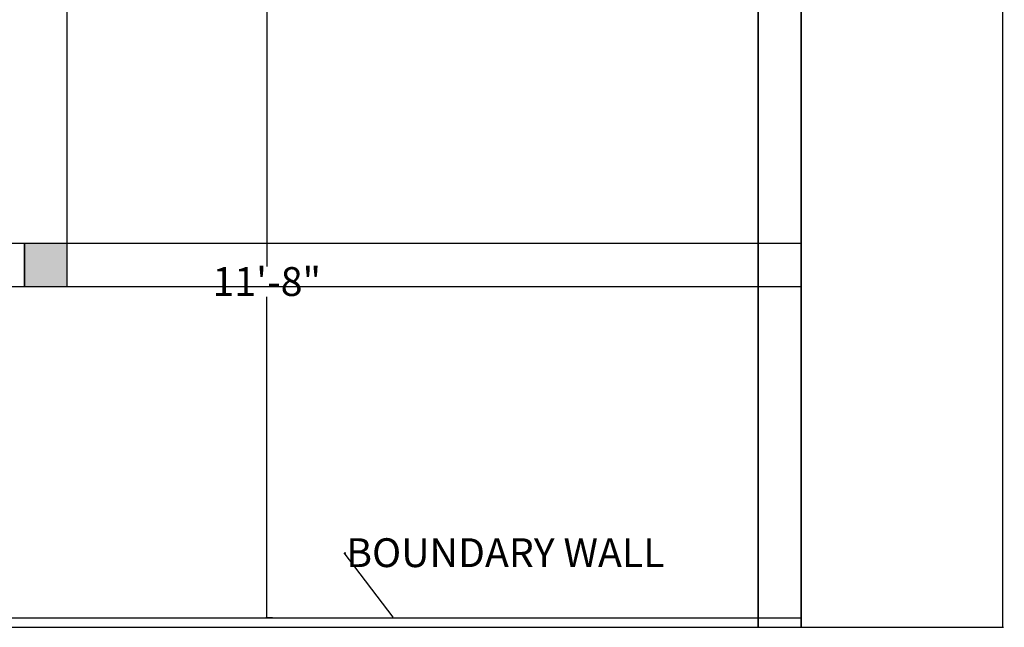
# Model space of a CAD drawing. Units: inches. Extents: x -36302355 to 648, y -221479757 to 75.
# Tile 14 of 37: x 442 to 647, y -722 to -595. Entities that reach past the tile are written whole.
import ezdxf
from ezdxf import colors
from ezdxf.entities.mleader import LeaderData, LeaderLine
from ezdxf.math import Vec2, Vec3

# ---------------------------------------------------------------- set-up
doc = ezdxf.new("R2010")
doc.units = ezdxf.units.IN
doc.header["$MEASUREMENT"] = 0
for name, color, linetype, lineweight in [('A-ANNO-DIMS', 2, 'Continuous', 18), ('A-ANNO-TEXT', 7, 'Continuous', 18), ('A-COLS', 7, 'Continuous', 35), ('A-COLS-PATT', 242, 'Continuous', 13), ('A-FLOR', 8, 'Continuous', 25), ('A-WALL', 7, 'Continuous', 35), ('L-WALL', 7, 'Continuous', 30)]:
    doc.layers.add(name, color=color, linetype=linetype, lineweight=lineweight)
doc.styles.get("Standard").update_dxf_attribs({"font": 'arial.ttf'})
doc.dimstyles.get("Standard").update_dxf_attribs({"dimtxt": 0.18, "dimasz": 0.18, "dimexe": 0.18, "dimexo": 0.0625, "dimgap": 0.09, "dimtad": 0, "dimtih": 1, "dimtoh": 1, "dimdec": 0, "dimzin": 0, "dimdsep": 46, "dimlunit": 3, "dimtxsty": 'Standard', "dimcen": 0.09, "dimadec": 0, "dimazin": 0, "dimtfac": 1, "dimtdec": 0, "dimtofl": 0, "dimtmove": 0, "dimatfit": 3, "dimfxl": 1, "dimtolj": 1, "dimtzin": 0, "dimarcsym": 0})

# ---------------------------------------------------------------- blocks, each defined once
blk = doc.blocks.new('*D8')
at = {"layer": 'A-ANNO-DIMS', "color": 0, "lineweight": -2, "transparency": 16777216}
for p, q in [((495.03, -580.02), (493.69, -580.02)), ((493.87, -580.2), (493.87, -646.87)), ((493.87, -719.84), (493.87, -653.17)), ((495.03, -720.02), (493.69, -720.02))]:
    blk.add_line(p, q, dxfattribs=at)
at = {"layer": 'A-ANNO-DIMS', "color": 0, "transparency": 16777216}
for points in [[(493.84, -580.2), (493.9, -580.2), (493.87, -580.02)], [(493.84, -719.84), (493.9, -719.84), (493.87, -720.02)]]:
    blk.add_solid(points, dxfattribs=at)
at = {"layer": 'Defpoints', "color": 0, "transparency": 16777216}
for p in [(495.09, -580.02), (493.87, -720.02), (495.09, -720.02)]:
    blk.add_point(p, dxfattribs=at)
at = {"layer": 'A-ANNO-DIMS', "color": 0, "transparency": 16777216, "insert": (493.87, -650.02), "char_height": 6, "attachment_point": 5}
blk.add_mtext('\\A1;11\'-8"', dxfattribs=at)
blk = doc.blocks.new('*D57')
at = {"layer": 'A-ANNO-DIMS', "color": 0, "lineweight": -2, "transparency": 16777216}
for p, q in [((605.26, 24.98), (647.33, 24.98)), ((647.15, 24.8), (647.15, -348.34)), ((647.15, -721.84), (647.15, -348.7)), ((605.26, -722.02), (647.33, -722.02))]:
    blk.add_line(p, q, dxfattribs=at)
at = {"layer": 'A-ANNO-DIMS', "color": 0, "transparency": 16777216}
for points in [[(647.12, 24.8), (647.18, 24.8), (647.15, 24.98)], [(647.12, -721.84), (647.18, -721.84), (647.15, -722.02)]]:
    blk.add_solid(points, dxfattribs=at)
at = {"layer": 'Defpoints', "color": 0, "transparency": 16777216}
for p in [(605.2, 24.98), (605.2, -722.02), (647.15, -722.02)]:
    blk.add_point(p, dxfattribs=at)
at = {"layer": 'A-ANNO-DIMS', "color": 0, "transparency": 16777216, "insert": (647.15, -348.52), "char_height": 0.18, "attachment_point": 5}
blk.add_mtext('\\A1;62\'-3"', dxfattribs=at)

msp = doc.modelspace()

# ---------------------------------------------------------------- hatches: boundary and pattern name
at = {"layer": 'A-COLS-PATT'}
h = msp.add_hatch(color=256, dxfattribs=at)
h.dxf.hatch_style = 1
h.paths.add_polyline_path([(283.54, -642.02), (274.2, -642.02), (274.2, -651.02), (283.54, -651.02)])
h.paths.add_polyline_path([(452.2, -642.02), (443.43, -642.02), (443.43, -651.02), (452.2, -651.02)])

# ---------------------------------------------------------------- linework, layer by layer
at = {"layer": 'A-COLS'}
msp.add_line((443.43, -642.02), (443.43, -651.02), dxfattribs=at)
at = {"layer": 'A-FLOR'}
for p, q in [((452.2, -580.02), (452.2, -651.02)), ((274.2, -642.02), (605.2, -642.02)), ((274.2, -651.02), (605.2, -651.02))]:
    msp.add_line(p, q, dxfattribs=at)
at = {"layer": 'A-WALL'}
for p, q in [((605.2, 24.98), (605.2, -722.02)), ((596.2, -431.02), (596.2, -722.02))]:
    msp.add_line(p, q, dxfattribs=at)
at = {"layer": 'L-WALL'}
for p, q in [((274.2, -720.02), (605.2, -720.02)), ((145.2, -722.02), (605.2, -722.02))]:
    msp.add_line(p, q, dxfattribs=at)

# ---------------------------------------------------------------- dimensions: what is measured, and where the dimension line sits
at = {"layer": 'A-ANNO-DIMS'}
for base, p1, p2, override, picture, middle in [((647.15, -722.02), (605.2, 24.98), (605.2, -722.02), {"dimdec": 1, "dimlfac": 1, "dimrnd": 0, "dimzin": 1, "dimdsep": 46, "dimlunit": 4, "dimfrac": 2}, '*D57', (647.15, -348.52)), ((493.87, -720.02), (495.09, -580.02), (495.09, -720.02), {"dimtxt": 6, "dimclrd": 0, "dimclre": 0, "dimclrt": 0}, '*D8', (493.87, -650.02))]:
    dim = msp.add_linear_dim(base=base, p1=p1, p2=p2, angle=90, dimstyle='Standard', override=override, dxfattribs=at)
    dim.commit()
    dim.dimension.update_dxf_attribs({"geometry": picture, "text_midpoint": middle})

# ---------------------------------------------------------------- leaders
at = {"layer": 'A-ANNO-TEXT'}
ml = msp.add_multileader_mtext('Standard', dxfattribs=at)
ml.set_content('BOUNDARY WALL', color=256)
ml.set_leader_properties()
ml.build(insert=Vec2(0, 0))
ml.multileader.update_dxf_attribs({"dogleg_length": 0.36, "arrow_head_size": 0.18})
ctx = ml.context
ctx.base_point, ctx.char_height, ctx.arrow_head_size, ctx.landing_gap_size, ctx.plane_origin = Vec3(510.32, -706.53), 6, 0.18, 0.09, Vec3(520.27, -720.02)
notes = []
notes.append((ctx, [(0, (1, 1, 0), (509.96, -706.53), (1, 0), 0.36, [(0, [(520.27, -720.02)], 0, [])])]))
ctx.mtext.insert, ctx.mtext.flow_direction = Vec3(510.41, -703.48), 5
for ctx, leaders in notes:
    for number, flags, end, landing, length, lines in leaders:
        leader = LeaderData()
        leader.index, (leader.has_last_leader_line, leader.has_dogleg_vector, leader.attachment_direction) = number, flags
        leader.last_leader_point, leader.dogleg_vector, leader.dogleg_length = Vec3(end), Vec3(landing), length
        for number, points, colour, breaks in lines:
            line = LeaderLine()
            line.index, line.vertices, line.color, line.breaks = number, Vec3.list(points), colors.encode_raw_color(colour), breaks
            leader.lines.append(line)
        ctx.leaders.append(leader)

doc.saveas('drawing.dxf')
